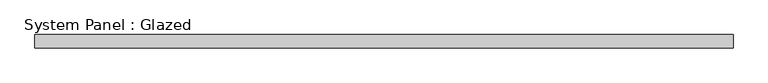
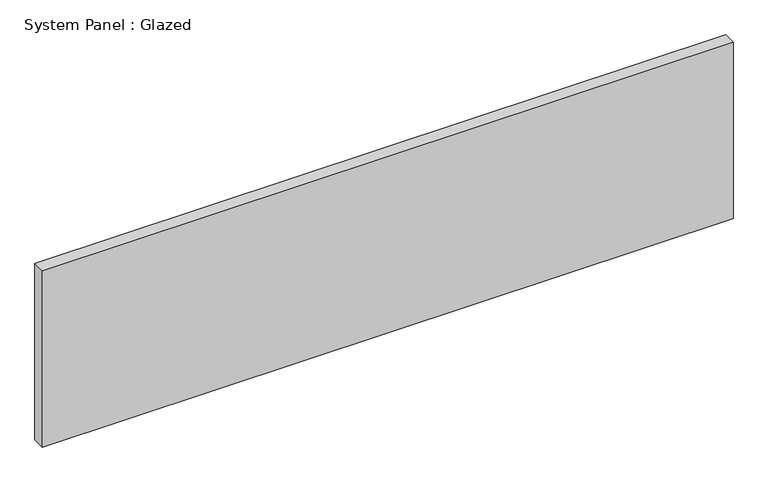
"""IFC4 building model written with IfcOpenShell, lengths in millimetres: plate geometry, System Panel : Glazed."""

from ifc_helpers import new_model, si_unit, origin, origin_with_axes, place, context, project, spatial, polyline, outline, extrude, source, transform, mapped, element, save


def system_panel_glazed_bee7dd50(model_context):
    return source(origin(), model_context, "Body", "SweptSolid", [
        extrude(outline(polyline([(669.9250001, 19.05), (-669.9250001, 19.05), (-669.9250001, 44.45), (669.9250001, 44.45), (669.9250001, 19.05)])), origin_with_axes(), (0.0, 0.0, 1.0), 361.95),
    ])


if __name__ == "__main__":
    model = new_model("IFC4")
    model_context = context("Model", 3, world=origin())
    ifc_project = project(units=[si_unit("LENGTHUNIT", "METRE", prefix="MILLI")], contexts=[model_context])
    site = spatial("IfcSite", under=ifc_project)
    building = spatial("IfcBuilding", under=site)
    placement = place(None, origin())
    system_panel_glazed_shape = system_panel_glazed_bee7dd50(model_context)
    element("IfcPlate", 1, ObjectType="System Panel : Glazed", at=placement, inside=building, context=model_context, shape_type="MappedRepresentation", body=[
        mapped(system_panel_glazed_shape, transform((0.0, 0.0, 0.0), x_axis=(1.0, 0.0, 0.0), y_axis=(0.0, 1.0, 0.0), z_axis=(0.0, 0.0, 1.0))),
    ])
    save(model, "model.ifc")

# Revit data of these elements
# Type "System Panel : Glazed"
#   Construction Type Id = "GSP4R"
#   Analytic Construction = "1/8 in Pilkington single glazing"
#   Visual Light Transmittance = 0.9
#   Solar Heat Gain Coefficient = 0.86
#   Heat Transfer Coefficient (U) = 1.18115 BTU/(h·ft²·°F)
#   Define Thermal Properties by = 1
# Element 1 (IfcPlate, "System Panel : Glazed")
#   Materials on its faces: "Glass"
# Materials
#   "Glass": class "Glass", colour RGB 0 128 192, transparency 0.75, Description = "Soda Lime Glass", Cost = 0
